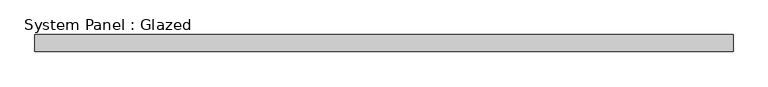
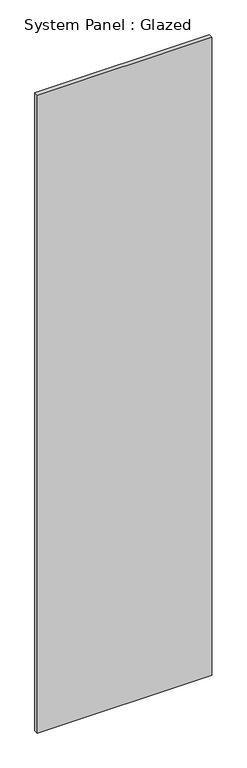
"""IFC4 building model written with IfcOpenShell, lengths in millimetres: plate geometry, System Panel : Glazed."""

from ifc_helpers import new_model, si_unit, origin, origin_with_axes, place, context, project, spatial, polyline, outline, extrude, source, transform, mapped, element, save


def system_panel_glazed_b430c16b(model_context):
    return source(origin(), model_context, "Body", "SweptSolid", [
        extrude(outline(polyline([(516.9735833, -49.5), (-516.9735833, -49.5), (-516.9735833, -24.5), (516.9735833, -24.5), (516.9735833, -49.5)])), origin_with_axes(), (0.0, 0.0, 1.0), 4000.0),
    ])


if __name__ == "__main__":
    model = new_model("IFC4")
    model_context = context("Model", 3, world=origin())
    ifc_project = project(units=[si_unit("LENGTHUNIT", "METRE", prefix="MILLI")], contexts=[model_context])
    site = spatial("IfcSite", under=ifc_project)
    building = spatial("IfcBuilding", under=site)
    placement = place(None, origin())
    system_panel_glazed_shape = system_panel_glazed_b430c16b(model_context)
    element("IfcPlate", 1, ObjectType="System Panel : Glazed", at=placement, inside=building, context=model_context, shape_type="MappedRepresentation", body=[
        mapped(system_panel_glazed_shape, transform((0.0, 0.0, 0.0), x_axis=(1.0, 0.0, 0.0), y_axis=(0.0, 1.0, 0.0), z_axis=(0.0, 0.0, 1.0))),
    ])
    save(model, "model.ifc")

# Revit data of these elements
# Type "System Panel : Glazed"
#   Keynote = "H11"
#   Construction Type Id = "GSP4R"
#   Analytic Construction = "1/8 in Pilkington single glazing"
#   Visual Light Transmittance = 0.9
#   Solar Heat Gain Coefficient = 0.86
#   Heat Transfer Coefficient (U) = 6.7069 W/(m²·K)
#   Define Thermal Properties by = 1
# Element 1 (IfcPlate, "System Panel : Glazed")
#   Materials on its faces: "Glass"
# Materials
#   "Glass": class "Glass", colour RGB 0 128 192, transparency 0.9, Description = "Soda Lime Glass", Cost = 0
